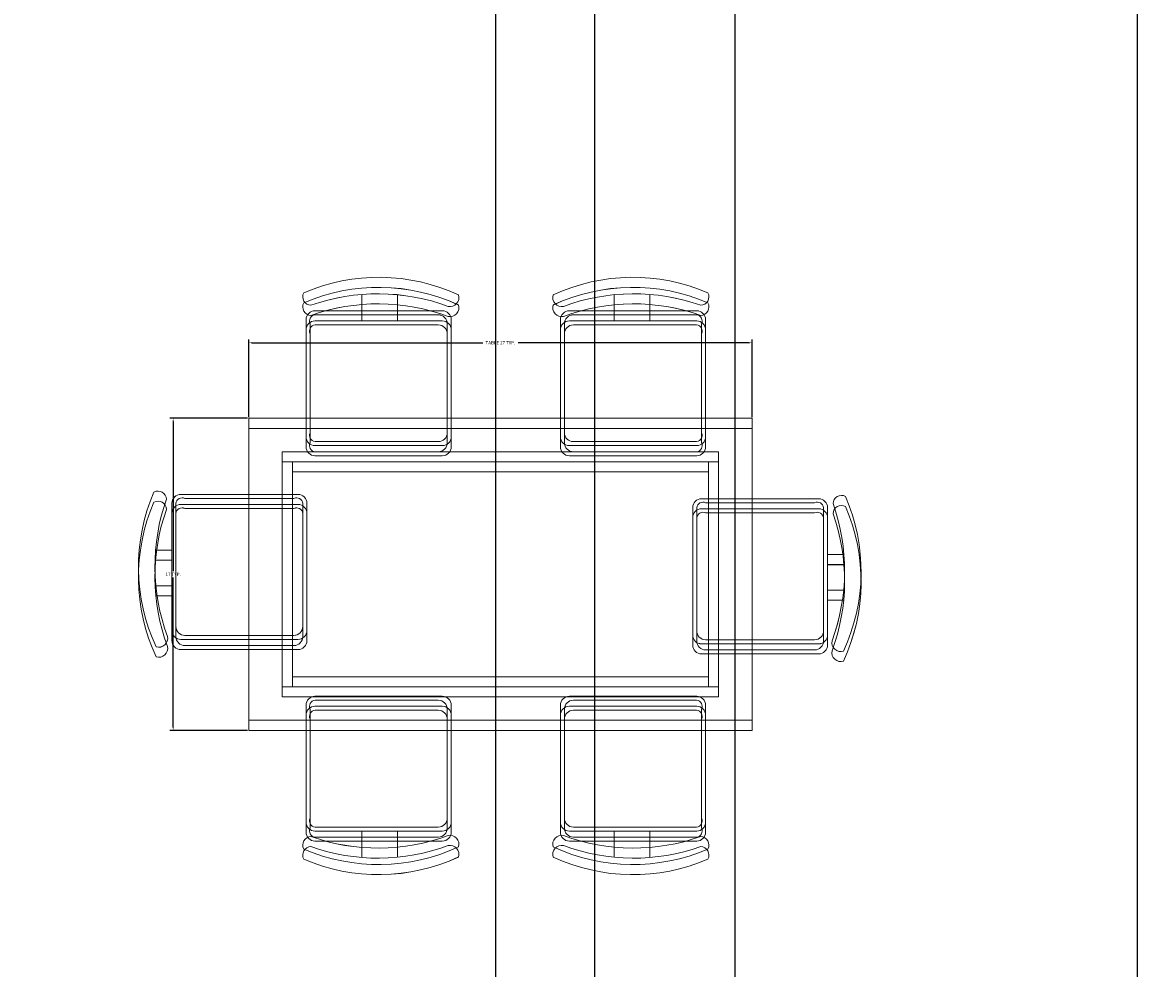
# Model space of a CAD drawing. Units: inches. Extents: x 2310 to 2937, y 1113 to 2410.
# Tile 4 of 23: x 2411 to 2472, y 1891 to 1943. Entities that reach past the tile are written whole.
import ezdxf

# ---------------------------------------------------------------- set-up
doc = ezdxf.new("R2010")
doc.units = ezdxf.units.IN
doc.layers.add('A-ANNO-DIMS', color=2, linetype='Continuous', lineweight=18)
doc.layers.add('A-FURN', color=8, linetype='Continuous', lineweight=18)
doc.styles.get("Standard").update_dxf_attribs({"font": 'arial.ttf'})
doc.dimstyles.get("Standard").update_dxf_attribs({"dimtxt": 0.18, "dimasz": 0.18, "dimexe": 0.18, "dimexo": 0.0625, "dimgap": 0.09, "dimtad": 0, "dimtih": 1, "dimtoh": 1, "dimdec": 4, "dimzin": 0, "dimdsep": 46, "dimtxsty": 'Standard', "dimcen": 0.09, "dimadec": 0, "dimazin": 0, "dimtfac": 1, "dimtdec": 4, "dimtofl": 0, "dimtmove": 0, "dimatfit": 3, "dimfxl": 1, "dimtolj": 1, "dimtzin": 0, "dimarcsym": 0})

# ---------------------------------------------------------------- blocks, each defined once
blk = doc.blocks.new('DINING-TABLE')
for points in [[(0, 17.017), (27.446, 17.017), (27.446, 0.549), (0, 0.549)], [(0, 17.016), (27.446, 17.016), (27.446, 0.549), (0, 0.549)], [(0, 16.468), (27.446, 16.468), (27.446, 0), (0, 0)], [(0, 16.467), (27.446, 16.467), (27.446, 0), (0, 0)], [(1.83, 15.187), (25.616, 15.187), (25.616, 2.379), (1.83, 2.379)], [(1.83, 15.187), (25.616, 15.187), (25.616, 2.379), (1.83, 2.379)], [(1.83, 14.638), (25.616, 14.638), (25.616, 1.83), (1.83, 1.83)], [(1.83, 14.638), (25.616, 14.638), (25.616, 1.83), (1.83, 1.83)], [(2.379, 14.638), (25.067, 14.638), (25.067, 2.928), (2.379, 2.928)], [(2.379, 14.638), (25.067, 14.638), (25.067, 2.928), (2.379, 2.928)], [(2.379, 14.089), (25.067, 14.089), (25.067, 2.379), (2.379, 2.379)], [(2.379, 14.089), (25.067, 14.089), (25.067, 2.379), (2.379, 2.379)]]:
    blk.add_lwpolyline(points, close=True)
blk = doc.blocks.new('CHAIR-DINING-2')
for points in [[(7.629, 2.699), (0.689, 2.699, -0.414214), (0.203, 3.185), (0.203, 9.566, -0.414214), (0.689, 10.052), (7.629, 10.052, -0.414214), (8.114, 9.566), (8.114, 3.185, -0.414214), (7.629, 2.699)], [(7.629, 2.699), (0.689, 2.699, -0.414214), (0.203, 3.185), (0.203, 9.566, -0.414214), (0.689, 10.051), (7.629, 10.051, -0.414214), (8.114, 9.566), (8.114, 3.185, -0.414214), (7.629, 2.699)], [(7.629, 2.15), (0.689, 2.15, -0.414214), (0.203, 2.636), (0.203, 9.017, -0.414214), (0.689, 9.503), (7.629, 9.503, -0.414214), (8.114, 9.017), (8.114, 2.636, -0.414214), (7.629, 2.15)], [(7.629, 2.15), (0.689, 2.15, -0.414214), (0.203, 2.636), (0.203, 9.017, -0.414214), (0.689, 9.502), (7.629, 9.502, -0.414214), (8.114, 9.017), (8.114, 2.636, -0.414214), (7.629, 2.15)], [(7.946, 2.456, -0.578392), (8.512, 1.833, -0.214524), (0.074, 1.72, -0.552014), (0.47, 2.399, 0.175809), (7.946, 2.456)], [(7.946, 2.456, -0.578392), (8.512, 1.833, -0.214524), (0.074, 1.72, -0.552014), (0.47, 2.399, 0.175809), (7.946, 2.456)], [(5.191, 2.699), (5.191, 1.822, 0.064759)], [(5.191, 2.699), (5.191, 1.821, 0.064759)], [(7.946, 1.907, -0.578392), (8.512, 1.284, -0.214524), (0.074, 1.171, -0.552014), (0.47, 1.85, 0.175809), (7.946, 1.907)], [(7.946, 1.907, -0.578392), (8.512, 1.284, -0.214524), (0.074, 1.171, -0.552014), (0.47, 1.85, 0.175809), (7.946, 1.907)], [(5.191, 2.15), (5.191, 1.273, 0.064759)], [(5.191, 2.15), (5.191, 1.272, 0.064759)]]:
    blk.add_lwpolyline(points, format="xyb")
for points in [[(0.692, 2.918), (7.41, 2.918, 0.414214), (7.895, 3.404), (7.895, 9.347, 0.414214), (7.41, 9.833), (0.692, 9.833, 0.512069), (0.422, 9.347), (0.422, 3.404, 0.512069)], [(0.692, 2.918), (7.41, 2.918, 0.414214), (7.895, 3.403), (7.895, 9.347, 0.414214), (7.41, 9.833), (0.692, 9.833, 0.512069), (0.422, 9.347), (0.422, 3.403, 0.512069)], [(0.692, 2.369), (7.41, 2.369, 0.414214), (7.895, 2.855), (7.895, 8.798, 0.414214), (7.41, 9.284), (0.692, 9.284, 0.512069), (0.422, 8.798), (0.422, 2.855, 0.512069)], [(0.692, 2.369), (7.41, 2.369, 0.414214), (7.895, 2.854), (7.895, 8.798, 0.414214), (7.41, 9.284), (0.692, 9.284, 0.512069), (0.422, 8.798), (0.422, 2.854, 0.512069)]]:
    blk.add_lwpolyline(points, format="xyb", close=True)
for points in [[(3.248, 1.806), (3.248, 2.699)], [(3.248, 1.805), (3.248, 2.699)], [(3.248, 1.257), (3.248, 2.15)], [(3.248, 1.257), (3.248, 2.15)]]:
    blk.add_lwpolyline(points)
blk = doc.blocks.new('CHAIR-DINING-3')
for points in [[(0.47, 8.201, -0.175809), (7.946, 8.145, 0.578392), (8.512, 8.768, 0.214524), (0.074, 8.881, 0.552014), (0.47, 8.201, -0.065079)], [(0.47, 8.201, -0.175809), (7.946, 8.145, 0.578392), (8.512, 8.767, 0.214524), (0.074, 8.88, 0.552014), (0.47, 8.201, -0.065079)], [(0.47, 7.653, -0.175809), (7.946, 7.596, 0.578392), (8.512, 8.219, 0.214524), (0.074, 8.332, 0.552014), (0.47, 7.653, -0.065079)], [(0.47, 7.652, -0.175809), (7.946, 7.596, 0.578392), (8.512, 8.218, 0.214524), (0.074, 8.332, 0.552014), (0.47, 7.652, -0.065079)], [(5.191, 7.901), (5.191, 8.779, -0.064759)], [(5.191, 7.901), (5.191, 8.779, -0.064759)], [(5.191, 7.352), (5.191, 8.23, -0.064759)], [(5.191, 7.352), (5.191, 8.23, -0.064759)], [(7.629, 7.901), (0.689, 7.901, 0.414214), (0.203, 7.416), (0.203, 1.035, 0.414214), (0.689, 0.549), (7.629, 0.549, 0.414214), (8.114, 1.035), (8.114, 7.416, 0.414214), (7.629, 7.901)], [(7.629, 7.901), (0.689, 7.901, 0.414214), (0.203, 7.416), (0.203, 1.034, 0.414214), (0.689, 0.549), (7.629, 0.549, 0.414214), (8.114, 1.034), (8.114, 7.416, 0.414214), (7.629, 7.901)], [(7.629, 7.352), (0.689, 7.352, 0.414214), (0.203, 6.867), (0.203, 0.486, 0.414214), (0.689, 0), (7.629, 0, 0.414214), (8.114, 0.486), (8.114, 6.867, 0.414214), (7.629, 7.352)], [(7.629, 7.352), (0.689, 7.352, 0.414214), (0.203, 6.867), (0.203, 0.486, 0.414214), (0.689, 0), (7.629, 0, 0.414214), (8.114, 0.486), (8.114, 6.867, 0.414214), (7.629, 7.352)]]:
    blk.add_lwpolyline(points, format="xyb")
for points in [[(3.248, 8.795), (3.248, 7.901)], [(3.248, 8.795), (3.248, 7.901)], [(3.248, 8.246), (3.248, 7.352)], [(3.248, 8.246), (3.248, 7.352)]]:
    blk.add_lwpolyline(points)
for points in [[(0.692, 7.683), (7.41, 7.683, -0.414214), (7.895, 7.197), (7.895, 1.253, -0.414214), (7.41, 0.768), (0.692, 0.768, -0.512069), (0.422, 1.253), (0.422, 7.197, -0.512069)], [(0.692, 7.682), (7.41, 7.682, -0.414214), (7.895, 7.197), (7.895, 1.253, -0.414214), (7.41, 0.768), (0.692, 0.768, -0.512069), (0.422, 1.253), (0.422, 7.197, -0.512069)], [(0.692, 7.134), (7.41, 7.134, -0.414214), (7.895, 6.648), (7.895, 0.705, -0.414214), (7.41, 0.219), (0.692, 0.219, -0.512069), (0.422, 0.705), (0.422, 6.648, -0.512069)], [(0.692, 7.133), (7.41, 7.133, -0.414214), (7.895, 6.648), (7.895, 0.704, -0.414214), (7.41, 0.219), (0.692, 0.219, -0.512069), (0.422, 0.704), (0.422, 6.648, -0.512069)]]:
    blk.add_lwpolyline(points, format="xyb", close=True)
blk = doc.blocks.new('CHAIR-DINING-4')
for points in [[(0.619, 8.145, -0.578392), (0.053, 8.768, -0.214524), (8.491, 8.881, -0.552014), (8.095, 8.201, 0.175809), (0.619, 8.145)], [(0.619, 8.145, -0.578392), (0.053, 8.767, -0.214524), (8.491, 8.88, -0.552014), (8.095, 8.201, 0.175809), (0.619, 8.145)], [(0.619, 7.596, -0.578392), (0.053, 8.219, -0.214524), (8.491, 8.332, -0.552014), (8.095, 7.653, 0.175809), (0.619, 7.596)], [(0.619, 7.596, -0.578392), (0.053, 8.218, -0.214524), (8.491, 8.332, -0.552014), (8.095, 7.652, 0.175809), (0.619, 7.596)], [(3.374, 7.901), (3.374, 8.779, 0.064759)], [(3.374, 7.901), (3.374, 8.779, 0.064759)], [(3.374, 7.352), (3.374, 8.23, 0.064759)], [(3.374, 7.352), (3.374, 8.23, 0.064759)], [(7.877, 7.901, -0.414214), (8.362, 7.416), (8.362, 1.035, -0.414214), (7.877, 0.549), (0.937, 0.549, -0.414214), (0.451, 1.035), (0.451, 7.416, -0.414214), (0.937, 7.901), (7.877, 7.901)], [(7.877, 7.901, -0.414214), (8.362, 7.416), (8.362, 1.034, -0.414214), (7.877, 0.549), (0.937, 0.549, -0.414214), (0.451, 1.034), (0.451, 7.416, -0.414214), (0.937, 7.901), (7.877, 7.901)], [(7.877, 7.352, -0.414214), (8.362, 6.867), (8.362, 0.486, -0.414214), (7.877, 0), (0.937, 0, -0.414214), (0.451, 0.486), (0.451, 6.867, -0.414214), (0.937, 7.352), (7.877, 7.352)], [(7.877, 7.352, -0.414214), (8.362, 6.867), (8.362, 0.486, -0.414214), (7.877, 0), (0.937, 0, -0.414214), (0.451, 0.486), (0.451, 6.867, -0.414214), (0.937, 7.352), (7.877, 7.352)]]:
    blk.add_lwpolyline(points, format="xyb")
for points in [[(5.317, 8.795), (5.317, 7.901)], [(5.317, 8.795), (5.317, 7.901)], [(5.317, 8.246), (5.317, 7.352)], [(5.317, 8.246), (5.317, 7.352)]]:
    blk.add_lwpolyline(points)
for points in [[(7.874, 7.683), (1.155, 7.683, 0.414214), (0.67, 7.197), (0.67, 1.253, 0.414214), (1.155, 0.768), (7.874, 0.768, 0.512069), (8.143, 1.253), (8.143, 7.197, 0.512069)], [(7.874, 7.682), (1.155, 7.682, 0.414214), (0.67, 7.197), (0.67, 1.253, 0.414214), (1.155, 0.768), (7.874, 0.768, 0.512069), (8.143, 1.253), (8.143, 7.197, 0.512069)], [(7.874, 7.134), (1.155, 7.134, 0.414214), (0.67, 6.648), (0.67, 0.705, 0.414214), (1.155, 0.219), (7.874, 0.219, 0.512069), (8.143, 0.705), (8.143, 6.648, 0.512069)], [(7.874, 7.133), (1.155, 7.133, 0.414214), (0.67, 6.648), (0.67, 0.704, 0.414214), (1.155, 0.219), (7.874, 0.219, 0.512069), (8.143, 0.704), (8.143, 6.648, 0.512069)]]:
    blk.add_lwpolyline(points, format="xyb", close=True)
blk = doc.blocks.new('CHAIR-DINING-6')
for points in [[(7.877, 2.699, 0.414214), (8.362, 3.185), (8.362, 9.566, 0.414214), (7.877, 10.052), (0.937, 10.052, 0.414214), (0.451, 9.566), (0.451, 3.185, 0.414214), (0.937, 2.699), (7.877, 2.699)], [(7.877, 2.699, 0.414214), (8.362, 3.185), (8.362, 9.566, 0.414214), (7.877, 10.051), (0.937, 10.051, 0.414214), (0.451, 9.566), (0.451, 3.185, 0.414214), (0.937, 2.699), (7.877, 2.699)], [(7.877, 2.15, 0.414214), (8.362, 2.636), (8.362, 9.017, 0.414214), (7.877, 9.503), (0.937, 9.503, 0.414214), (0.451, 9.017), (0.451, 2.636, 0.414214), (0.937, 2.15), (7.877, 2.15)], [(7.877, 2.15, 0.414214), (8.362, 2.636), (8.362, 9.017, 0.414214), (7.877, 9.502), (0.937, 9.502, 0.414214), (0.451, 9.017), (0.451, 2.636, 0.414214), (0.937, 2.15), (7.877, 2.15)], [(8.095, 2.399, -0.175809), (0.619, 2.456, 0.578392), (0.053, 1.833, 0.214524), (8.491, 1.72, 0.552014), (8.095, 2.399, -0.065079)], [(8.095, 2.399, -0.175809), (0.619, 2.456, 0.578392), (0.053, 1.833, 0.214524), (8.491, 1.72, 0.552014), (8.095, 2.399, -0.065079)], [(3.374, 2.699), (3.374, 1.822, -0.064759)], [(3.374, 2.699), (3.374, 1.821, -0.064759)], [(8.095, 1.85, -0.175809), (0.619, 1.907, 0.578392), (0.053, 1.284, 0.214524), (8.491, 1.171, 0.552014), (8.095, 1.85, -0.065079)], [(8.095, 1.85, -0.175809), (0.619, 1.907, 0.578392), (0.053, 1.284, 0.214524), (8.491, 1.171, 0.552014), (8.095, 1.85, -0.065079)], [(3.374, 2.15), (3.374, 1.273, -0.064759)], [(3.374, 2.15), (3.374, 1.272, -0.064759)]]:
    blk.add_lwpolyline(points, format="xyb")
for points in [[(7.874, 2.918), (1.155, 2.918, -0.414214), (0.67, 3.404), (0.67, 9.347, -0.414214), (1.155, 9.833), (7.874, 9.833, -0.512069), (8.143, 9.347), (8.143, 3.404, -0.512069)], [(7.874, 2.918), (1.155, 2.918, -0.414214), (0.67, 3.403), (0.67, 9.347, -0.414214), (1.155, 9.833), (7.874, 9.833, -0.512069), (8.143, 9.347), (8.143, 3.403, -0.512069)], [(7.874, 2.369), (1.155, 2.369, -0.414214), (0.67, 2.855), (0.67, 8.798, -0.414214), (1.155, 9.284), (7.874, 9.284, -0.512069), (8.143, 8.798), (8.143, 2.855, -0.512069)], [(7.874, 2.369), (1.155, 2.369, -0.414214), (0.67, 2.854), (0.67, 8.798, -0.414214), (1.155, 9.284), (7.874, 9.284, -0.512069), (8.143, 8.798), (8.143, 2.854, -0.512069)]]:
    blk.add_lwpolyline(points, format="xyb", close=True)
for points in [[(5.317, 1.806), (5.317, 2.699)], [(5.317, 1.805), (5.317, 2.699)], [(5.317, 1.257), (5.317, 2.15)], [(5.317, 1.257), (5.317, 2.15)]]:
    blk.add_lwpolyline(points)
blk = doc.blocks.new('*D17')
at = {"layer": 'A-ANNO-DIMS', "color": 0, "lineweight": -2, "transparency": 16777216}
for p, q in [((2423.008, 1921.333), (2423.008, 1925.567)), ((2423.188, 1925.387), (2435.768, 1925.387)), ((2450.274, 1925.387), (2437.695, 1925.387)), ((2450.454, 1921.333), (2450.454, 1925.567))]:
    blk.add_line(p, q, dxfattribs=at)
at = {"layer": 'A-ANNO-DIMS', "color": 0, "transparency": 16777216}
for points in [[(2423.188, 1925.417), (2423.188, 1925.357), (2423.008, 1925.387)], [(2450.274, 1925.417), (2450.274, 1925.357), (2450.454, 1925.387)]]:
    blk.add_solid(points, dxfattribs=at)
at = {"layer": 'Defpoints', "color": 0, "transparency": 16777216}
for p in [(2450.454, 1925.387), (2423.008, 1921.27), (2450.454, 1921.27)]:
    blk.add_point(p, dxfattribs=at)
at = {"layer": 'A-ANNO-DIMS', "color": 0, "transparency": 16777216, "insert": (2436.731, 1925.387), "char_height": 0.18, "attachment_point": 5}
blk.add_mtext('\\A1;TABLE 27 TYP.', dxfattribs=at)
blk = doc.blocks.new('*D18')
at = {"layer": 'A-ANNO-DIMS', "color": 0, "lineweight": -2, "transparency": 16777216}
for p, q in [((2422.946, 1921.27), (2418.712, 1921.27)), ((2418.892, 1921.09), (2418.892, 1912.942)), ((2418.892, 1904.434), (2418.892, 1912.581)), ((2422.946, 1904.254), (2418.712, 1904.254))]:
    blk.add_line(p, q, dxfattribs=at)
at = {"layer": 'A-ANNO-DIMS', "color": 0, "transparency": 16777216}
for points in [[(2418.862, 1921.09), (2418.922, 1921.09), (2418.892, 1921.27)], [(2418.862, 1904.434), (2418.922, 1904.434), (2418.892, 1904.254)]]:
    blk.add_solid(points, dxfattribs=at)
at = {"layer": 'Defpoints', "color": 0, "transparency": 16777216}
for p in [(2418.892, 1921.27), (2423.008, 1921.27), (2423.008, 1904.254)]:
    blk.add_point(p, dxfattribs=at)
at = {"layer": 'A-ANNO-DIMS', "color": 0, "transparency": 16777216, "insert": (2418.892, 1912.762), "char_height": 0.18, "attachment_point": 5}
blk.add_mtext('\\A1;17 TYP.', dxfattribs=at)
blk = doc.blocks.new('*D60')
at = {"layer": 'A-ANNO-DIMS', "color": 0, "lineweight": -2, "transparency": 16777216}
for p, q in [((2449.502, 2205.951), (2449.502, 1649.501)), ((2471.439, 2205.951), (2471.439, 1649.501)), ((2449.682, 1649.681), (2460.005, 1649.681)), ((2471.259, 1649.681), (2460.936, 1649.681))]:
    blk.add_line(p, q, dxfattribs=at)
at = {"layer": 'A-ANNO-DIMS', "color": 0, "transparency": 16777216}
for points in [[(2449.682, 1649.711), (2449.682, 1649.651), (2449.502, 1649.681)], [(2471.259, 1649.711), (2471.259, 1649.651), (2471.439, 1649.681)]]:
    blk.add_solid(points, dxfattribs=at)
at = {"layer": 'Defpoints', "color": 0, "transparency": 16777216}
for p in [(2449.502, 2206.014), (2471.439, 2206.014), (2471.439, 1649.681)]:
    blk.add_point(p, dxfattribs=at)
at = {"layer": 'A-ANNO-DIMS', "color": 0, "transparency": 16777216, "insert": (2460.471, 1649.681), "char_height": 0.18, "attachment_point": 5}
blk.add_mtext('\\A1;21.936', dxfattribs=at)
blk = doc.blocks.new('*D63')
at = {"layer": 'A-ANNO-DIMS', "color": 0, "lineweight": -2, "transparency": 16777216}
for p, q in [((2436.465, 1999.451), (2436.465, 1649.501)), ((2524.465, 1999.451), (2524.465, 1649.501)), ((2436.645, 1649.681), (2480.245, 1649.681)), ((2524.285, 1649.681), (2480.684, 1649.681))]:
    blk.add_line(p, q, dxfattribs=at)
at = {"layer": 'A-ANNO-DIMS', "color": 0, "transparency": 16777216}
for points in [[(2436.645, 1649.711), (2436.645, 1649.651), (2436.465, 1649.681)], [(2524.285, 1649.711), (2524.285, 1649.651), (2524.465, 1649.681)]]:
    blk.add_solid(points, dxfattribs=at)
at = {"layer": 'Defpoints', "color": 0, "transparency": 16777216}
for p in [(2436.465, 1999.514), (2524.465, 1999.514), (2524.465, 1649.681)]:
    blk.add_point(p, dxfattribs=at)
at = {"layer": 'A-ANNO-DIMS', "color": 0, "transparency": 16777216, "insert": (2480.465, 1649.681), "char_height": 0.18, "attachment_point": 5}
blk.add_mtext('\\A1;88', dxfattribs=at)
blk = doc.blocks.new('*D65')
at = {"layer": 'A-ANNO-DIMS', "color": 0, "lineweight": -2, "transparency": 16777216}
for p, q in [((2403.486, 2093.451), (2403.486, 1649.501)), ((2436.465, 2093.451), (2436.465, 1649.501)), ((2403.666, 1649.681), (2419.581, 1649.681)), ((2436.285, 1649.681), (2420.369, 1649.681))]:
    blk.add_line(p, q, dxfattribs=at)
at = {"layer": 'A-ANNO-DIMS', "color": 0, "transparency": 16777216}
for points in [[(2403.666, 1649.711), (2403.666, 1649.651), (2403.486, 1649.681)], [(2436.285, 1649.711), (2436.285, 1649.651), (2436.465, 1649.681)]]:
    blk.add_solid(points, dxfattribs=at)
at = {"layer": 'Defpoints', "color": 0, "transparency": 16777216}
for p in [(2403.486, 2093.514), (2436.465, 2093.514), (2436.465, 1649.681)]:
    blk.add_point(p, dxfattribs=at)
at = {"layer": 'A-ANNO-DIMS', "color": 0, "transparency": 16777216, "insert": (2419.975, 1649.681), "char_height": 0.18, "attachment_point": 5}
blk.add_mtext('\\A1;32.98', dxfattribs=at)
blk = doc.blocks.new('*D69')
at = {"layer": 'A-ANNO-DIMS', "color": 0, "lineweight": -2, "transparency": 16777216}
for p, q in [((2441.861, 2131.962), (2441.861, 1649.501)), ((2475.893, 2131.962), (2475.893, 1649.501)), ((2442.041, 1649.681), (2458.483, 1649.681)), ((2475.713, 1649.681), (2459.271, 1649.681))]:
    blk.add_line(p, q, dxfattribs=at)
at = {"layer": 'A-ANNO-DIMS', "color": 0, "transparency": 16777216}
for points in [[(2442.041, 1649.711), (2442.041, 1649.651), (2441.861, 1649.681)], [(2475.713, 1649.711), (2475.713, 1649.651), (2475.893, 1649.681)]]:
    blk.add_solid(points, dxfattribs=at)
at = {"layer": 'Defpoints', "color": 0, "transparency": 16777216}
for p in [(2441.861, 2132.024), (2475.893, 2132.024), (2475.893, 1649.681)]:
    blk.add_point(p, dxfattribs=at)
at = {"layer": 'A-ANNO-DIMS', "color": 0, "transparency": 16777216, "insert": (2458.877, 1649.681), "char_height": 0.18, "attachment_point": 5}
blk.add_mtext('\\A1;34.03', dxfattribs=at)

msp = doc.modelspace()

# ---------------------------------------------------------------- linework, layer by layer
at = {"layer": 'A-FURN'}
for points in [[(2426.4032, 1927.4312, -0.1758092), (2433.8786, 1927.3746, 0.5783921), (2434.4449, 1927.9973, 0.2145244), (2426.0068, 1928.1106, 0.552014), (2426.4032, 1927.4312, -0.065079)], [(2426.4032, 1927.4309, -0.1758092), (2433.8786, 1927.3743, 0.5783921), (2434.445, 1927.9971, 0.2145244), (2426.0068, 1928.1103, 0.552014), (2426.4032, 1927.4309, -0.065079)], [(2426.4032, 1926.8823, -0.1758092), (2433.8786, 1926.8257, 0.5783921), (2434.4449, 1927.4484, 0.2145244), (2426.0068, 1927.5616, 0.552014), (2426.4032, 1926.8823, -0.065079)], [(2426.4032, 1926.882, -0.1758092), (2433.8786, 1926.8254, 0.5783921), (2434.445, 1927.4481, 0.2145244), (2426.0068, 1927.5614, 0.552014), (2426.4032, 1926.882, -0.065079)], [(2431.1238, 1927.1312), (2431.1238, 1928.0089, -0.0647586)], [(2431.1238, 1927.1309), (2431.1238, 1928.0086, -0.0647586)], [(2431.1238, 1926.5823), (2431.1238, 1927.46, -0.0647586)], [(2431.1238, 1926.582), (2431.1238, 1927.4597, -0.0647586)], [(2433.5615, 1927.1312), (2426.6215, 1927.1312, 0.4142136), (2426.136, 1926.6457), (2426.136, 1920.2645, 0.4142136), (2426.6215, 1919.779), (2433.5615, 1919.779, 0.4142136), (2434.047, 1920.2645), (2434.047, 1926.6457, 0.4142136), (2433.5615, 1927.1312)], [(2433.5615, 1927.1309), (2426.6215, 1927.1309, 0.4142136), (2426.136, 1926.6454), (2426.136, 1920.2642, 0.4142136), (2426.6215, 1919.7787), (2433.5615, 1919.7787, 0.4142136), (2434.047, 1920.2642), (2434.047, 1926.6454, 0.4142136), (2433.5615, 1927.1309)], [(2433.5615, 1926.5823), (2426.6215, 1926.5823, 0.4142136), (2426.136, 1926.0968), (2426.136, 1919.7156, 0.4142136), (2426.6215, 1919.2301), (2433.5615, 1919.2301, 0.4142136), (2434.047, 1919.7156), (2434.047, 1926.0968, 0.4142136), (2433.5615, 1926.5823)], [(2433.5615, 1926.582), (2426.6215, 1926.582, 0.4142136), (2426.136, 1926.0965), (2426.136, 1919.7153, 0.4142136), (2426.6215, 1919.2298), (2433.5615, 1919.2298, 0.4142136), (2434.047, 1919.7153), (2434.047, 1926.0965, 0.4142136), (2433.5615, 1926.582)], [(2418.5824, 1909.3792, -0.5783921), (2417.9597, 1908.8129, -0.2145244), (2417.8465, 1917.2511, -0.552014), (2418.5258, 1916.8546, 0.1758094), (2418.5824, 1909.3792)], [(2418.5824, 1909.3792, -0.5783921), (2417.9597, 1908.8129, -0.2145244), (2417.8465, 1917.2511, -0.552014), (2418.5258, 1916.8546, 0.1758094), (2418.5824, 1909.3792)], [(2418.5825, 1909.3789, -0.5783921), (2417.9597, 1908.8126, -0.2145244), (2417.8465, 1917.2508, -0.552014), (2418.5258, 1916.8543, 0.1758094), (2418.5825, 1909.3789)], [(2418.5825, 1909.3789, -0.5783921), (2417.9597, 1908.8126, -0.2145244), (2417.8465, 1917.2508, -0.552014), (2418.5258, 1916.8543, 0.1758094), (2418.5825, 1909.3789)], [(2418.8259, 1916.6363, -0.4142136), (2419.3114, 1917.1218), (2425.6925, 1917.1218, -0.4142136), (2426.1781, 1916.6363), (2426.1781, 1909.6963, -0.4142136), (2425.6925, 1909.2108), (2419.3114, 1909.2108, -0.4142136), (2418.8259, 1909.6963), (2418.8259, 1916.6363)], [(2418.8259, 1916.6363, -0.4142136), (2419.3114, 1917.1218), (2425.6925, 1917.1218, -0.4142136), (2426.1781, 1916.6363), (2426.1781, 1909.6963, -0.4142136), (2425.6925, 1909.2108), (2419.3114, 1909.2108, -0.4142136), (2418.8259, 1909.6963), (2418.8259, 1916.6363)], [(2418.8259, 1916.636, -0.4142136), (2419.3114, 1917.1215), (2425.6925, 1917.1215, -0.4142136), (2426.1781, 1916.636), (2426.1781, 1909.6961, -0.4142136), (2425.6925, 1909.2105), (2419.3114, 1909.2105, -0.4142136), (2418.8259, 1909.6961), (2418.8259, 1916.636)], [(2418.8259, 1916.636, -0.4142136), (2419.3114, 1917.1215), (2425.6925, 1917.1215, -0.4142136), (2426.1781, 1916.636), (2426.1781, 1909.6961, -0.4142136), (2425.6925, 1909.2105), (2419.3114, 1909.2105, -0.4142136), (2418.8259, 1909.6961), (2418.8259, 1916.636)], [(2454.8633, 1916.6169, -0.1758092), (2454.8067, 1909.1415, 0.5783921), (2455.4295, 1908.5752, 0.2145244), (2455.5427, 1917.0134, 0.552014), (2454.8633, 1916.6169, -0.065079)], [(2454.8633, 1916.6169, -0.1758092), (2454.8067, 1909.1415, 0.5783921), (2455.4295, 1908.5752, 0.2145244), (2455.5427, 1917.0134, 0.552014), (2454.8633, 1916.6169, -0.065079)], [(2454.8634, 1916.6167, -0.1758092), (2454.8068, 1909.1412, 0.5783921), (2455.4295, 1908.5749, 0.2145244), (2455.5427, 1917.0131, 0.552014), (2454.8634, 1916.6167, -0.065079)], [(2454.8634, 1916.6167, -0.1758092), (2454.8068, 1909.1412, 0.5783921), (2455.4295, 1908.5749, 0.2145244), (2455.5427, 1917.0131, 0.552014), (2454.8634, 1916.6167, -0.065079)], [(2418.5824, 1908.8303, -0.5783921), (2417.9597, 1908.264, -0.2145244), (2417.8465, 1916.7021, -0.552014), (2418.5258, 1916.3057, 0.1758094), (2418.5824, 1908.8303)], [(2418.5824, 1908.8303, -0.5783921), (2417.9597, 1908.264, -0.2145244), (2417.8465, 1916.7021, -0.552014), (2418.5258, 1916.3057, 0.1758094), (2418.5824, 1908.8303)], [(2418.5825, 1908.83, -0.5783921), (2417.9597, 1908.2637, -0.2145244), (2417.8465, 1916.7018, -0.552014), (2418.5258, 1916.3054, 0.1758094), (2418.5825, 1908.83)], [(2418.5825, 1908.83, -0.5783921), (2417.9597, 1908.2637, -0.2145244), (2417.8465, 1916.7018, -0.552014), (2418.5258, 1916.3054, 0.1758094), (2418.5825, 1908.83)], [(2418.8259, 1916.0874, -0.4142136), (2419.3114, 1916.5729), (2425.6925, 1916.5729, -0.4142136), (2426.1781, 1916.0874), (2426.1781, 1909.1474, -0.4142136), (2425.6925, 1908.6619), (2419.3114, 1908.6619, -0.4142136), (2418.8259, 1909.1474), (2418.8259, 1916.0874)], [(2418.8259, 1916.0874, -0.4142136), (2419.3114, 1916.5729), (2425.6925, 1916.5729, -0.4142136), (2426.1781, 1916.0874), (2426.1781, 1909.1474, -0.4142136), (2425.6925, 1908.6619), (2419.3114, 1908.6619, -0.4142136), (2418.8259, 1909.1474), (2418.8259, 1916.0874)], [(2418.8259, 1916.0871, -0.4142136), (2419.3114, 1916.5726), (2425.6925, 1916.5726, -0.4142136), (2426.1781, 1916.0871), (2426.1781, 1909.1471, -0.4142136), (2425.6925, 1908.6616), (2419.3114, 1908.6616, -0.4142136), (2418.8259, 1909.1471), (2418.8259, 1916.0871)], [(2418.8259, 1916.0871, -0.4142136), (2419.3114, 1916.5726), (2425.6925, 1916.5726, -0.4142136), (2426.1781, 1916.0871), (2426.1781, 1909.1471, -0.4142136), (2425.6925, 1908.6616), (2419.3114, 1908.6616, -0.4142136), (2418.8259, 1909.1471), (2418.8259, 1916.0871)], [(2454.5633, 1916.3986, 0.4142136), (2454.0778, 1916.8841), (2447.6966, 1916.8841, 0.4142136), (2447.2111, 1916.3986), (2447.2111, 1909.4587, 0.4142136), (2447.6966, 1908.9731), (2454.0778, 1908.9731, 0.4142136), (2454.5633, 1909.4587), (2454.5633, 1916.3986)], [(2454.5633, 1916.3986, 0.4142136), (2454.0778, 1916.8841), (2447.6966, 1916.8841, 0.4142136), (2447.2111, 1916.3986), (2447.2111, 1909.4587, 0.4142136), (2447.6966, 1908.9731), (2454.0778, 1908.9731, 0.4142136), (2454.5633, 1909.4587), (2454.5633, 1916.3986)], [(2454.5633, 1916.3983, 0.4142136), (2454.0778, 1916.8838), (2447.6967, 1916.8838, 0.4142136), (2447.2111, 1916.3983), (2447.2111, 1909.4584, 0.4142136), (2447.6967, 1908.9728), (2454.0778, 1908.9728, 0.4142136), (2454.5633, 1909.4584), (2454.5633, 1916.3983)], [(2454.5633, 1916.3983, 0.4142136), (2454.0778, 1916.8838), (2447.6967, 1916.8838, 0.4142136), (2447.2111, 1916.3983), (2447.2111, 1909.4584, 0.4142136), (2447.6967, 1908.9728), (2454.0778, 1908.9728, 0.4142136), (2454.5633, 1909.4584), (2454.5633, 1916.3983)], [(2454.8633, 1916.068, -0.1758092), (2454.8067, 1908.5926, 0.5783921), (2455.4295, 1908.0263, 0.2145244), (2455.5427, 1916.4645, 0.552014), (2454.8633, 1916.068, -0.065079)], [(2454.8633, 1916.068, -0.1758092), (2454.8067, 1908.5926, 0.5783921), (2455.4295, 1908.0263, 0.2145244), (2455.5427, 1916.4645, 0.552014), (2454.8633, 1916.068, -0.065079)], [(2454.8634, 1916.0677, -0.1758092), (2454.8068, 1908.5923, 0.5783921), (2455.4295, 1908.026, 0.2145244), (2455.5427, 1916.4642, 0.552014), (2454.8634, 1916.0677, -0.065079)], [(2454.8634, 1916.0677, -0.1758092), (2454.8068, 1908.5923, 0.5783921), (2455.4295, 1908.026, 0.2145244), (2455.5427, 1916.4642, 0.552014), (2454.8634, 1916.0677, -0.065079)], [(2454.5633, 1915.8497, 0.4142136), (2454.0778, 1916.3352), (2447.6966, 1916.3352, 0.4142136), (2447.2111, 1915.8497), (2447.2111, 1908.9097, 0.4142136), (2447.6966, 1908.4242), (2454.0778, 1908.4242, 0.4142136), (2454.5633, 1908.9097), (2454.5633, 1915.8497)], [(2454.5633, 1915.8497, 0.4142136), (2454.0778, 1916.3352), (2447.6966, 1916.3352, 0.4142136), (2447.2111, 1915.8497), (2447.2111, 1908.9097, 0.4142136), (2447.6966, 1908.4242), (2454.0778, 1908.4242, 0.4142136), (2454.5633, 1908.9097), (2454.5633, 1915.8497)], [(2454.5633, 1915.8494, 0.4142136), (2454.0778, 1916.3349), (2447.6967, 1916.3349, 0.4142136), (2447.2111, 1915.8494), (2447.2111, 1908.9095, 0.4142136), (2447.6967, 1908.4239), (2454.0778, 1908.4239, 0.4142136), (2454.5633, 1908.9095), (2454.5633, 1915.8494)], [(2454.5633, 1915.8494, 0.4142136), (2454.0778, 1916.3349), (2447.6967, 1916.3349, 0.4142136), (2447.2111, 1915.8494), (2447.2111, 1908.9095, 0.4142136), (2447.6967, 1908.4239), (2454.0778, 1908.4239, 0.4142136), (2454.5633, 1908.9095), (2454.5633, 1915.8494)], [(2418.8259, 1912.134), (2417.9482, 1912.134, 0.0647586)], [(2418.8259, 1912.134), (2417.9482, 1912.134, 0.0647586)], [(2418.8259, 1912.1337), (2417.9482, 1912.1337, 0.0647586)], [(2418.8259, 1912.1337), (2417.9482, 1912.1337, 0.0647586)], [(2418.8259, 1911.5851), (2417.9482, 1911.5851, 0.0647586)], [(2418.8259, 1911.5851), (2417.9482, 1911.5851, 0.0647586)], [(2418.8259, 1911.5848), (2417.9482, 1911.5848, 0.0647586)], [(2418.8259, 1911.5848), (2417.9482, 1911.5848, 0.0647586)], [(2454.5633, 1911.8963), (2455.441, 1911.8963, -0.0647586)], [(2454.5633, 1911.8963), (2455.441, 1911.8963, -0.0647586)], [(2454.5633, 1911.896), (2455.441, 1911.896, -0.0647586)], [(2454.5633, 1911.896), (2455.441, 1911.896, -0.0647586)], [(2454.5633, 1911.3474), (2455.441, 1911.3474, -0.0647586)], [(2454.5633, 1911.3474), (2455.441, 1911.3474, -0.0647586)], [(2454.5633, 1911.3471), (2455.441, 1911.3471, -0.0647586)], [(2454.5633, 1911.3471), (2455.441, 1911.3471, -0.0647586)], [(2433.5615, 1898.7655), (2426.6215, 1898.7655, -0.4142136), (2426.136, 1899.251), (2426.136, 1905.6321, -0.4142136), (2426.6215, 1906.1177), (2433.5615, 1906.1177, -0.4142136), (2434.047, 1905.6321), (2434.047, 1899.251, -0.4142136), (2433.5615, 1898.7655)], [(2433.5615, 1898.7655), (2426.6215, 1898.7655, -0.4142136), (2426.136, 1899.251), (2426.136, 1905.6321, -0.4142136), (2426.6215, 1906.1177), (2433.5615, 1906.1177, -0.4142136), (2434.047, 1905.6321), (2434.047, 1899.251, -0.4142136), (2433.5615, 1898.7655)], [(2433.5615, 1898.7652), (2426.6215, 1898.7652, -0.4142136), (2426.136, 1899.2507), (2426.136, 1905.6318, -0.4142136), (2426.6215, 1906.1174), (2433.5615, 1906.1174, -0.4142136), (2434.047, 1905.6318), (2434.047, 1899.2507, -0.4142136), (2433.5615, 1898.7652)], [(2433.5615, 1898.7652), (2426.6215, 1898.7652, -0.4142136), (2426.136, 1899.2507), (2426.136, 1905.6318, -0.4142136), (2426.6215, 1906.1174), (2433.5615, 1906.1174, -0.4142136), (2434.047, 1905.6318), (2434.047, 1899.2507, -0.4142136), (2433.5615, 1898.7652)], [(2433.5615, 1898.2165), (2426.6215, 1898.2165, -0.4142136), (2426.136, 1898.7021), (2426.136, 1905.0832, -0.4142136), (2426.6215, 1905.5687), (2433.5615, 1905.5687, -0.4142136), (2434.047, 1905.0832), (2434.047, 1898.7021, -0.4142136), (2433.5615, 1898.2165)], [(2433.5615, 1898.2165), (2426.6215, 1898.2165, -0.4142136), (2426.136, 1898.7021), (2426.136, 1905.0832, -0.4142136), (2426.6215, 1905.5687), (2433.5615, 1905.5687, -0.4142136), (2434.047, 1905.0832), (2434.047, 1898.7021, -0.4142136), (2433.5615, 1898.2165)], [(2433.5615, 1898.2163), (2426.6215, 1898.2163, -0.4142136), (2426.136, 1898.7018), (2426.136, 1905.0829, -0.4142136), (2426.6215, 1905.5685), (2433.5615, 1905.5685, -0.4142136), (2434.047, 1905.0829), (2434.047, 1898.7018, -0.4142136), (2433.5615, 1898.2163)], [(2433.5615, 1898.2163), (2426.6215, 1898.2163, -0.4142136), (2426.136, 1898.7018), (2426.136, 1905.0829, -0.4142136), (2426.6215, 1905.5685), (2433.5615, 1905.5685, -0.4142136), (2434.047, 1905.0829), (2434.047, 1898.7018, -0.4142136), (2433.5615, 1898.2163)], [(2433.8786, 1898.522, -0.5783921), (2434.4449, 1897.8993, -0.2145244), (2426.0068, 1897.7861, -0.552014), (2426.4032, 1898.4654, 0.1758093), (2433.8786, 1898.522)], [(2433.8786, 1898.522, -0.5783921), (2434.4449, 1897.8993, -0.2145244), (2426.0068, 1897.7861, -0.552014), (2426.4032, 1898.4654, 0.1758093), (2433.8786, 1898.522)], [(2433.8786, 1898.5217, -0.5783921), (2434.445, 1897.899, -0.2145244), (2426.0068, 1897.7858, -0.552014), (2426.4032, 1898.4651, 0.1758093), (2433.8786, 1898.5217)], [(2433.8786, 1898.5217, -0.5783921), (2434.445, 1897.899, -0.2145244), (2426.0068, 1897.7858, -0.552014), (2426.4032, 1898.4651, 0.1758093), (2433.8786, 1898.5217)], [(2431.1238, 1898.7655), (2431.1238, 1897.8878, 0.0647586)], [(2431.1238, 1898.7655), (2431.1238, 1897.8878, 0.0647586)], [(2431.1238, 1898.7652), (2431.1238, 1897.8875, 0.0647586)], [(2431.1238, 1898.7652), (2431.1238, 1897.8875, 0.0647586)], [(2433.8786, 1897.9731, -0.5783921), (2434.4449, 1897.3504, -0.2145244), (2426.0068, 1897.2372, -0.552014), (2426.4032, 1897.9165, 0.1758093), (2433.8786, 1897.9731)], [(2433.8786, 1897.9731, -0.5783921), (2434.4449, 1897.3504, -0.2145244), (2426.0068, 1897.2372, -0.552014), (2426.4032, 1897.9165, 0.1758093), (2433.8786, 1897.9731)], [(2433.8786, 1897.9728, -0.5783921), (2434.445, 1897.3501, -0.2145244), (2426.0068, 1897.2369, -0.552014), (2426.4032, 1897.9162, 0.1758093), (2433.8786, 1897.9728)], [(2433.8786, 1897.9728, -0.5783921), (2434.445, 1897.3501, -0.2145244), (2426.0068, 1897.2369, -0.552014), (2426.4032, 1897.9162, 0.1758093), (2433.8786, 1897.9728)], [(2431.1238, 1898.2165), (2431.1238, 1897.3389, 0.0647586)], [(2431.1238, 1898.2165), (2431.1238, 1897.3389, 0.0647586)], [(2431.1238, 1898.2163), (2431.1238, 1897.3386, 0.0647586)], [(2431.1238, 1898.2163), (2431.1238, 1897.3386, 0.0647586)]]:
    msp.add_lwpolyline(points, format="xyb", dxfattribs=at)
for points in [[(2429.1812, 1928.0248), (2429.1812, 1927.1312)], [(2429.1812, 1928.0246), (2429.1812, 1927.1309)], [(2429.1812, 1927.4759), (2429.1812, 1926.5823)], [(2429.1812, 1927.4756), (2429.1812, 1926.582)], [(2417.9322, 1914.0766), (2418.8259, 1914.0766)], [(2417.9322, 1914.0766), (2418.8259, 1914.0766)], [(2417.9322, 1914.0763), (2418.8259, 1914.0763)], [(2417.9322, 1914.0763), (2418.8259, 1914.0763)], [(2417.9322, 1913.5277), (2418.8259, 1913.5277)], [(2417.9322, 1913.5277), (2418.8259, 1913.5277)], [(2417.9322, 1913.5274), (2418.8259, 1913.5274)], [(2417.9322, 1913.5274), (2418.8259, 1913.5274)], [(2455.457, 1913.8389), (2454.5633, 1913.8389)], [(2455.457, 1913.8389), (2454.5633, 1913.8389)], [(2455.457, 1913.8386), (2454.5633, 1913.8386)], [(2455.457, 1913.8386), (2454.5633, 1913.8386)], [(2455.457, 1913.29), (2454.5633, 1913.29)], [(2455.457, 1913.29), (2454.5633, 1913.29)], [(2455.457, 1913.2897), (2454.5633, 1913.2897)], [(2455.457, 1913.2897), (2454.5633, 1913.2897)], [(2429.1812, 1897.8718), (2429.1812, 1898.7655)], [(2429.1812, 1897.8718), (2429.1812, 1898.7655)], [(2429.1812, 1897.8715), (2429.1812, 1898.7652)], [(2429.1812, 1897.8715), (2429.1812, 1898.7652)], [(2429.1812, 1897.3229), (2429.1812, 1898.2165)], [(2429.1812, 1897.3229), (2429.1812, 1898.2165)], [(2429.1812, 1897.3226), (2429.1812, 1898.2163)], [(2429.1812, 1897.3226), (2429.1812, 1898.2163)]]:
    msp.add_lwpolyline(points, dxfattribs=at)
for points in [[(2426.6245, 1926.9125), (2433.3427, 1926.9125, -0.4142136), (2433.8283, 1926.4269), (2433.8283, 1920.4833, -0.4142136), (2433.3427, 1919.9977), (2426.6245, 1919.9977, -0.5120695), (2426.3547, 1920.4833), (2426.3547, 1926.4269, -0.5120695)], [(2426.6245, 1926.9122), (2433.3428, 1926.9122, -0.4142136), (2433.8283, 1926.4267), (2433.8283, 1920.483, -0.4142136), (2433.3428, 1919.9975), (2426.6245, 1919.9975, -0.5120695), (2426.3547, 1920.483), (2426.3547, 1926.4267, -0.5120695)], [(2426.6245, 1926.3636), (2433.3427, 1926.3636, -0.4142136), (2433.8283, 1925.878), (2433.8283, 1919.9344, -0.4142136), (2433.3427, 1919.4488), (2426.6245, 1919.4488, -0.5120695), (2426.3547, 1919.9344), (2426.3547, 1925.878, -0.5120695)], [(2426.6245, 1926.3633), (2433.3428, 1926.3633, -0.4142136), (2433.8283, 1925.8777), (2433.8283, 1919.9341, -0.4142136), (2433.3428, 1919.4485), (2426.6245, 1919.4485, -0.5120695), (2426.3547, 1919.9341), (2426.3547, 1925.8777, -0.5120695)], [(2419.0446, 1916.6333), (2419.0446, 1909.9151, 0.4142136), (2419.5301, 1909.4295), (2425.4738, 1909.4295, 0.4142136), (2425.9593, 1909.9151), (2425.9593, 1916.6333, 0.5120695), (2425.4738, 1916.9031), (2419.5301, 1916.9031, 0.5120695)], [(2419.0446, 1916.6333), (2419.0446, 1909.9151, 0.4142136), (2419.5301, 1909.4295), (2425.4738, 1909.4295, 0.4142136), (2425.9593, 1909.9151), (2425.9593, 1916.6333, 0.5120695), (2425.4738, 1916.9031), (2419.5301, 1916.9031, 0.5120695)], [(2419.0446, 1916.633), (2419.0446, 1909.9148, 0.4142136), (2419.5301, 1909.4293), (2425.4738, 1909.4293, 0.4142136), (2425.9593, 1909.9148), (2425.9593, 1916.633, 0.5120695), (2425.4738, 1916.9028), (2419.5301, 1916.9028, 0.5120695)], [(2419.0446, 1916.633), (2419.0446, 1909.9148, 0.4142136), (2419.5301, 1909.4293), (2425.4738, 1909.4293, 0.4142136), (2425.9593, 1909.9148), (2425.9593, 1916.633, 0.5120695), (2425.4738, 1916.9028), (2419.5301, 1916.9028, 0.5120695)], [(2419.0446, 1916.0844), (2419.0446, 1909.3662, 0.4142136), (2419.5301, 1908.8806), (2425.4738, 1908.8806, 0.4142136), (2425.9593, 1909.3662), (2425.9593, 1916.0844, 0.5120695), (2425.4738, 1916.3542), (2419.5301, 1916.3542, 0.5120695)], [(2419.0446, 1916.0844), (2419.0446, 1909.3662, 0.4142136), (2419.5301, 1908.8806), (2425.4738, 1908.8806, 0.4142136), (2425.9593, 1909.3662), (2425.9593, 1916.0844, 0.5120695), (2425.4738, 1916.3542), (2419.5301, 1916.3542, 0.5120695)], [(2419.0446, 1916.0841), (2419.0446, 1909.3659, 0.4142136), (2419.5301, 1908.8803), (2425.4738, 1908.8803, 0.4142136), (2425.9593, 1909.3659), (2425.9593, 1916.0841, 0.5120695), (2425.4738, 1916.3539), (2419.5301, 1916.3539, 0.5120695)], [(2419.0446, 1916.0841), (2419.0446, 1909.3659, 0.4142136), (2419.5301, 1908.8803), (2425.4738, 1908.8803, 0.4142136), (2425.9593, 1909.3659), (2425.9593, 1916.0841, 0.5120695), (2425.4738, 1916.3539), (2419.5301, 1916.3539, 0.5120695)], [(2454.3446, 1916.3957), (2454.3446, 1909.6774, -0.4142136), (2453.8591, 1909.1919), (2447.9154, 1909.1919, -0.4142136), (2447.4299, 1909.6774), (2447.4299, 1916.3957, -0.5120695), (2447.9154, 1916.6654), (2453.8591, 1916.6654, -0.5120695)], [(2454.3446, 1916.3957), (2454.3446, 1909.6774, -0.4142136), (2453.8591, 1909.1919), (2447.9154, 1909.1919, -0.4142136), (2447.4299, 1909.6774), (2447.4299, 1916.3957, -0.5120695), (2447.9154, 1916.6654), (2453.8591, 1916.6654, -0.5120695)], [(2454.3446, 1916.3954), (2454.3446, 1909.6771, -0.4142136), (2453.8591, 1909.1916), (2447.9154, 1909.1916, -0.4142136), (2447.4299, 1909.6771), (2447.4299, 1916.3954, -0.5120695), (2447.9154, 1916.6651), (2453.8591, 1916.6651, -0.5120695)], [(2454.3446, 1916.3954), (2454.3446, 1909.6771, -0.4142136), (2453.8591, 1909.1916), (2447.9154, 1909.1916, -0.4142136), (2447.4299, 1909.6771), (2447.4299, 1916.3954, -0.5120695), (2447.9154, 1916.6651), (2453.8591, 1916.6651, -0.5120695)], [(2454.3446, 1915.8467), (2454.3446, 1909.1285, -0.4142136), (2453.8591, 1908.643), (2447.9154, 1908.643, -0.4142136), (2447.4299, 1909.1285), (2447.4299, 1915.8467, -0.5120695), (2447.9154, 1916.1165), (2453.8591, 1916.1165, -0.5120695)], [(2454.3446, 1915.8467), (2454.3446, 1909.1285, -0.4142136), (2453.8591, 1908.643), (2447.9154, 1908.643, -0.4142136), (2447.4299, 1909.1285), (2447.4299, 1915.8467, -0.5120695), (2447.9154, 1916.1165), (2453.8591, 1916.1165, -0.5120695)], [(2454.3446, 1915.8465), (2454.3446, 1909.1282, -0.4142136), (2453.8591, 1908.6427), (2447.9154, 1908.6427, -0.4142136), (2447.4299, 1909.1282), (2447.4299, 1915.8465, -0.5120695), (2447.9154, 1916.1162), (2453.8591, 1916.1162, -0.5120695)], [(2454.3446, 1915.8465), (2454.3446, 1909.1282, -0.4142136), (2453.8591, 1908.6427), (2447.9154, 1908.6427, -0.4142136), (2447.4299, 1909.1282), (2447.4299, 1915.8465, -0.5120695), (2447.9154, 1916.1162), (2453.8591, 1916.1162, -0.5120695)], [(2426.6245, 1898.9842), (2433.3427, 1898.9842, 0.4142136), (2433.8283, 1899.4697), (2433.8283, 1905.4134, 0.4142136), (2433.3427, 1905.8989), (2426.6245, 1905.8989, 0.5120695), (2426.3547, 1905.4134), (2426.3547, 1899.4697, 0.5120695)], [(2426.6245, 1898.9842), (2433.3427, 1898.9842, 0.4142136), (2433.8283, 1899.4697), (2433.8283, 1905.4134, 0.4142136), (2433.3427, 1905.8989), (2426.6245, 1905.8989, 0.5120695), (2426.3547, 1905.4134), (2426.3547, 1899.4697, 0.5120695)], [(2426.6245, 1898.9839), (2433.3428, 1898.9839, 0.4142136), (2433.8283, 1899.4694), (2433.8283, 1905.4131, 0.4142136), (2433.3428, 1905.8986), (2426.6245, 1905.8986, 0.5120695), (2426.3547, 1905.4131), (2426.3547, 1899.4694, 0.5120695)], [(2426.6245, 1898.9839), (2433.3428, 1898.9839, 0.4142136), (2433.8283, 1899.4694), (2433.8283, 1905.4131, 0.4142136), (2433.3428, 1905.8986), (2426.6245, 1905.8986, 0.5120695), (2426.3547, 1905.4131), (2426.3547, 1899.4694, 0.5120695)], [(2426.6245, 1898.4353), (2433.3427, 1898.4353, 0.4142136), (2433.8283, 1898.9208), (2433.8283, 1904.8645, 0.4142136), (2433.3427, 1905.35), (2426.6245, 1905.35, 0.5120695), (2426.3547, 1904.8645), (2426.3547, 1898.9208, 0.5120695)], [(2426.6245, 1898.4353), (2433.3427, 1898.4353, 0.4142136), (2433.8283, 1898.9208), (2433.8283, 1904.8645, 0.4142136), (2433.3427, 1905.35), (2426.6245, 1905.35, 0.5120695), (2426.3547, 1904.8645), (2426.3547, 1898.9208, 0.5120695)], [(2426.6245, 1898.435), (2433.3428, 1898.435, 0.4142136), (2433.8283, 1898.9205), (2433.8283, 1904.8642, 0.4142136), (2433.3428, 1905.3497), (2426.6245, 1905.3497, 0.5120695), (2426.3547, 1904.8642), (2426.3547, 1898.9205, 0.5120695)], [(2426.6245, 1898.435), (2433.3428, 1898.435, 0.4142136), (2433.8283, 1898.9205), (2433.8283, 1904.8642, 0.4142136), (2433.3428, 1905.3497), (2426.6245, 1905.3497, 0.5120695), (2426.3547, 1904.8642), (2426.3547, 1898.9205, 0.5120695)]]:
    msp.add_lwpolyline(points, format="xyb", close=True, dxfattribs=at)

# ---------------------------------------------------------------- block references
for name, p in [('CHAIR-DINING-3', (2425.9329, 1919.2298)), ('CHAIR-DINING-4', (2439.5525, 1919.2298)), ('DINING-TABLE', (2423.0084, 1904.2536)), ('DINING-TABLE', (2423.0084, 1904.2536)), ('CHAIR-DINING-6', (2439.5525, 1896.0661)), ('CHAIR-DINING-6', (2439.5525, 1896.0661))]:
    msp.add_blockref(name, p, dxfattribs=at)
at = {"layer": 'A-FURN', "rotation": 180}
msp.add_blockref('CHAIR-DINING-2', (2448.1177, 1929.2814), dxfattribs=at)

# ---------------------------------------------------------------- dimensions: what is measured, and where the dimension line sits
at = {"layer": 'A-ANNO-DIMS'}
for base, p1, p2, override, picture, middle in [((2471.4388, 1649.6807), (2449.5024, 2206.0139), (2471.4388, 2206.0139), {"dimdec": 3, "dimlfac": 1, "dimrnd": 0, "dimzin": 0, "dimdsep": 46, "dimlunit": 2}, '*D60', (2460.4706, 1649.6807)), ((2475.8929, 1649.6807), (2441.8613, 2132.0241), (2475.8929, 2132.0241), {"dimdec": 2, "dimlfac": 1, "dimrnd": 0, "dimzin": 0, "dimdsep": 46, "dimlunit": 2}, '*D69', (2458.8771, 1649.6807)), ((2436.4647, 1649.6807), (2403.4859, 2093.5139), (2436.4647, 2093.5139), {"dimdec": 2, "dimlfac": 1, "dimrnd": 0, "dimzin": 0, "dimdsep": 46, "dimlunit": 2}, '*D65', (2419.9753, 1649.6807)), ((2524.4647, 1649.6807), (2436.4647, 1999.5139), (2524.4647, 1999.5139), {"dimdec": 0, "dimlfac": 1, "dimrnd": 0, "dimzin": 0, "dimdsep": 46, "dimlunit": 2}, '*D63', (2480.4647, 1649.6807))]:
    dim = msp.add_linear_dim(base=base, p1=p1, p2=p2, dimstyle='Standard', override=override, dxfattribs=at)
    dim.commit()
    dim.dimension.update_dxf_attribs({"geometry": picture, "text_midpoint": middle})
dim = msp.add_linear_dim(base=(2450.4542, 1925.3871), p1=(2423.0084, 1921.2702), p2=(2450.4542, 1921.2702), text='TABLE <> TYP.', dimstyle='Standard', override={"dimdec": 0, "dimlfac": 1, "dimrnd": 0, "dimzin": 0, "dimdsep": 46, "dimlunit": 2}, dxfattribs=at)
dim.commit()
dim.dimension.update_dxf_attribs({"geometry": '*D17', "text_midpoint": (2436.7313, 1925.3871)})
dim = msp.add_linear_dim(base=(2418.8916, 1921.2702), p1=(2423.0084, 1904.2536), p2=(2423.0084, 1921.2702), angle=90, text='<> TYP.', dimstyle='Standard', override={"dimdec": 0, "dimlfac": 1, "dimrnd": 0, "dimzin": 0, "dimdsep": 46, "dimlunit": 2}, dxfattribs=at)
dim.commit()
dim.dimension.update_dxf_attribs({"geometry": '*D18', "text_midpoint": (2418.8916, 1912.7619)})

doc.saveas('drawing.dxf')
